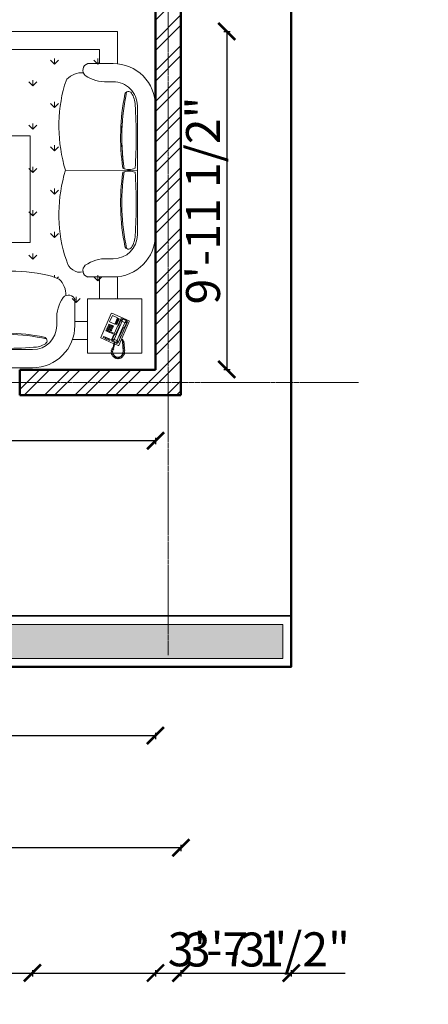
# Model space of a CAD drawing. Units: inches. Extents: x 261 to 2725, y 291 to 1454.
# Tile 11 of 35: x 898 to 1043, y 293 to 641. Entities that reach past the tile are written whole.
import ezdxf

# ---------------------------------------------------------------- set-up
doc = ezdxf.new("R2010")
doc.units = ezdxf.units.IN
doc.linetypes.add('CENTER', pattern=[2, 1.25, -0.25, 0.25, -0.25])
for name, color, linetype, lineweight in [('A-ANNO-DIMS', 136, 'Continuous', 18), ('A-FURN', 30, 'Continuous', 18), ('A-GRID', 251, 'CENTER', 13), ('A-PLNT', 3, 'Continuous', 18), ('A-PLNT-PATT', 3, 'Continuous', 13), ('A-WALL', 222, 'Continuous', 50), ('A-WALL-PATT', 243, 'Continuous', 13), ('C-PROP', 7, 'Continuous', 35)]:
    doc.layers.add(name, color=color, linetype=linetype, lineweight=lineweight)
doc.styles.get("Standard").update_dxf_attribs({"font": 'arial.ttf'})
doc.dimstyles.new('ISO-25', dxfattribs={"dimtxt": 12, "dimasz": 6, "dimexe": 1.25, "dimexo": 0.625, "dimtad": 1, "dimdec": 0, "dimlunit": 3, "dimtxsty": 'Standard', "dimblk": 'ARCHTICK', "dimcen": 2.5, "dimadec": 0, "dimazin": 0, "dimtfac": 1, "dimtdec": 0, "dimtmove": 0, "dimatfit": 3, "dimfxl": 1, "dimfxlon": 1, "dimarcsym": 0})

# ---------------------------------------------------------------- blocks, each defined once
blk = doc.blocks.new('A$C29956593')
for p, q in [((1017.8, 2786), (2742.6, 2786)), ((278.2, 2702.6), (273.3, 2697.8)), ((273.3, 2697.8), (276.9, 2686.9)), ((285.5, 2696.3), (278.2, 2702.6)), ((283.9, 2691.1), (302.3, 2697.9)), ((290.3, 2707.8), (284.9, 2706)), ((284.9, 2706), (285.5, 2696.3)), ((296.9, 2700.7), (290.3, 2707.8)), ((303.3, 2712.1), (296.9, 2710.1)), ((296.9, 2710.1), (296.9, 2700.7)), ((302.3, 2697.9), (322.4, 2697.8)), ((306.1, 2701.8), (303.3, 2712.1)), ((309.1, 2711), (306.1, 2701.8)), ((314.8, 2711.2), (309.1, 2711)), ((318.9, 2702.4), (314.8, 2711.2)), ((322.6, 2710.2), (318.9, 2702.4)), ((322.4, 2697.8), (339.2, 2688.6)), ((328.8, 2709.2), (322.6, 2710.2)), ((327.9, 2698.5), (328.8, 2709.2)), ((333.7, 2706), (327.9, 2698.5)), ((338.4, 2703.2), (333.7, 2706)), ((338.4, 2693.8), (338.4, 2703.2)), ((345.6, 2700), (338.4, 2693.8)), ((351, 2695.6), (345.6, 2700)), ((345.9, 2686.3), (351, 2695.6)), ((869.5, 2753), (870.7, 2751.8)), ((113, 2666.3), (113, 2216.3)), ((563, 2666.3), (113, 2666.3)), ((255.7, 2654.1), (254.5, 2644.2)), ((254.5, 2644.2), (263.6, 2641.2)), ((263.6, 2641.2), (254.7, 2635.1)), ((254.7, 2635.1), (255.8, 2629)), ((265.6, 2653.6), (255.7, 2654.1)), ((255.8, 2629), (265, 2627.7)), ((257.1, 2665), (256.2, 2657.4)), ((256.2, 2657.4), (265.6, 2653.6)), ((265.8, 2668.1), (257.1, 2665)), ((265, 2627.7), (257.1, 2621.8)), ((257.1, 2621.8), (257.6, 2614.3)), ((257.6, 2614.3), (266.7, 2613.4)), ((259.7, 2679.5), (257.9, 2671.6)), ((257.9, 2671.6), (265.8, 2668.1)), ((266.7, 2613.4), (258.5, 2609)), ((269.9, 2678.1), (259.7, 2679.5)), ((268, 2691.2), (264.2, 2685.9)), ((264.2, 2685.9), (269.9, 2678.1)), ((267.7, 2639.4), (270.2, 2671)), ((269.6, 2618.4), (267.7, 2639.4)), ((267.7, 2616.4), (269.6, 2618.4)), ((269.4, 2615), (267.7, 2616.4)), ((276.9, 2686.9), (268, 2691.2)), ((270.3, 2600.3), (269.4, 2615)), ((270.2, 2671), (283.9, 2691.1)), ((339.2, 2688.6), (351, 2673.6)), ((345.1, 2616), (342.8, 2608.6)), ((349.3, 2635.7), (345.1, 2629.6)), ((345.1, 2629.6), (348.7, 2623.5)), ((348.7, 2623.5), (345.1, 2616)), ((355.4, 2689.1), (345.9, 2686.3)), ((346.5, 2598), (349, 2613.2)), ((349, 2613.2), (352.7, 2620.7)), ((355.9, 2654.7), (349.3, 2635.7)), ((351, 2673.6), (355.9, 2654.7)), ((352.6, 2622.8), (357.2, 2624.6)), ((352.7, 2620.7), (352.6, 2622.8)), ((353.1, 2636.5), (363.4, 2637.8)), ((360.9, 2631.3), (353.1, 2636.5)), ((354.8, 2675.8), (359.4, 2683.1)), ((363.7, 2677.8), (354.8, 2675.8)), ((359.4, 2683.1), (355.4, 2689.1)), ((357.2, 2624.6), (360.9, 2631.3)), ((357.4, 2651), (368.4, 2653.8)), ((366.3, 2646), (357.4, 2651)), ((358, 2664.3), (365.7, 2670.6)), ((367.5, 2662.1), (358, 2664.3)), ((363.4, 2637.8), (366.3, 2646)), ((365.7, 2670.6), (363.7, 2677.8)), ((368.4, 2653.8), (367.5, 2662.1)), ((563, 2216.3), (563, 2666.3)), ((2910.7, 2636), (1017.8, 2636)), ((216.6, 2403), (304.3, 2601.6)), ((231.9, 2406.6), (308.2, 2579.2)), ((258.5, 2609), (258.5, 2601.3)), ((258.5, 2601.3), (267.9, 2601.3)), ((267.9, 2601.3), (258.9, 2597.3)), ((258.9, 2597.3), (259.1, 2591.7)), ((259.1, 2591.7), (268.7, 2590.5)), ((268.7, 2590.5), (260.3, 2584.2)), ((260.3, 2584.2), (260.7, 2578.8)), ((260.7, 2578.8), (269.3, 2577.7)), ((261.3, 2572.2), (261.1, 2568.5)), ((261.1, 2568.5), (263.9, 2566.2)), ((269.3, 2577.7), (261.3, 2572.2)), ((263.9, 2566.2), (269, 2563.6)), ((269, 2563.6), (270.6, 2556.3)), ((269.2, 2568), (274, 2569.4)), ((272.1, 2566.8), (269.2, 2568)), ((272.6, 2580.5), (270.3, 2600.3)), ((270.6, 2556.3), (273.2, 2552.7)), ((273.1, 2564.2), (272.1, 2566.8)), ((274, 2569.4), (272.6, 2580.5)), ((275.7, 2559.9), (273.1, 2564.2)), ((273.2, 2552.7), (280.8, 2548.3)), ((277.9, 2556.2), (275.7, 2559.9)), ((282.7, 2552.6), (277.9, 2556.2)), ((283.4, 2480.1), (317.7, 2557.8)), ((365, 2555.9), (288, 2381.8)), ((293.3, 2537.7), (293, 2529.2)), ((310.5, 2576.5), (293.3, 2537.7)), ((304.3, 2601.6), (308.5, 2603.2)), ((306.4, 2470), (340.7, 2547.7)), ((308.2, 2579.2), (319.2, 2584.7)), ((308.5, 2603.2), (339.5, 2589.5)), ((314.4, 2581.6), (310.5, 2576.5)), ((310.5, 2576.5), (317.7, 2557.8)), ((321.5, 2581.9), (314.4, 2581.6)), ((317.7, 2557.8), (320.4, 2560.1)), ((319.2, 2584.7), (336.1, 2577.2)), ((320.4, 2560.1), (321.5, 2581.9)), ((320.4, 2560.1), (340.5, 2551.2)), ((335.5, 2575.7), (321.5, 2581.9)), ((338.2, 2583.2), (333.9, 2571.3)), ((333.9, 2571.3), (338.3, 2569.4)), ((340.3, 2593.4), (338.2, 2583.2)), ((338.3, 2569.4), (343.5, 2581.9)), ((356, 2566.7), (340.1, 2573.7)), ((342.8, 2608.6), (340.3, 2593.4)), ((340.5, 2551.2), (356, 2566.7)), ((340.7, 2547.7), (340.5, 2551.2)), ((340.7, 2575.2), (360.9, 2566.2)), ((359.4, 2554.9), (340.7, 2547.7)), ((359.4, 2554.9), (342.2, 2516)), ((343.5, 2581.9), (346.5, 2598)), ((344.5, 2587.2), (452.3, 2539.6)), ((356, 2566.7), (360.5, 2561.3)), ((360.5, 2561.3), (359.4, 2554.9)), ((360.9, 2566.2), (365, 2555.9)), ((453.9, 2535.4), (366.2, 2336.9)), ((378.8, 2560), (375, 2551.4)), ((375, 2551.4), (389.4, 2545)), ((393.2, 2553.7), (378.8, 2560)), ((389.4, 2545), (393.2, 2553.7)), ((399, 2551.1), (395.2, 2542.5)), ((395.2, 2542.5), (409.6, 2536.1)), ((413.4, 2544.8), (399, 2551.1)), ((409.6, 2536.1), (413.4, 2544.8)), ((419.1, 2542.2), (415.3, 2533.6)), ((415.3, 2533.6), (429.7, 2527.2)), ((433.5, 2535.9), (419.1, 2542.2)), ((429.7, 2527.2), (433.5, 2535.9)), ((452.3, 2539.6), (453.9, 2535.4)), ((688, 2553), (563, 2553)), ((253.3, 2447), (259.3, 2452.9)), ((283.4, 2480.1), (254.8, 2415.4)), ((259.3, 2452.9), (266.8, 2458.2)), ((266.8, 2458.2), (272.7, 2467.7)), ((272.7, 2467.7), (279, 2482.1)), ((306.4, 2470), (277.8, 2405.2)), ((291.1, 2509.4), (279, 2482.1)), ((294.1, 2520.1), (291.1, 2509.4)), ((293, 2529.2), (294.1, 2520.1)), ((301.3, 2443), (304.3, 2453.7)), ((304.3, 2453.7), (310.7, 2468.1)), ((322.8, 2495.4), (310.7, 2468.1)), ((328.7, 2504.8), (322.8, 2495.4)), ((336.2, 2510.1), (328.7, 2504.8)), ((342.2, 2516), (336.2, 2510.1)), ((348.6, 2441), (352.4, 2449.6)), ((349.4, 2497.4), (353.2, 2506)), ((360.9, 2492.3), (349.4, 2497.4)), ((352.4, 2449.6), (361, 2445.8)), ((353.2, 2506), (364.8, 2500.9)), ((355.6, 2456.8), (359.4, 2465.5)), ((364.2, 2453), (355.6, 2456.8)), ((359.4, 2465.5), (368, 2461.6)), ((364.8, 2500.9), (360.9, 2492.3)), ((362.6, 2472.7), (366.4, 2481.3)), ((371.2, 2468.8), (362.6, 2472.7)), ((368, 2461.6), (364.2, 2453)), ((366.4, 2481.3), (375, 2477.5)), ((369.6, 2488.5), (373.4, 2497.1)), ((378.2, 2484.7), (369.6, 2488.5)), ((370, 2450.5), (373.8, 2459.1)), ((378.6, 2446.7), (370, 2450.5)), ((375, 2477.5), (371.2, 2468.8)), ((373.4, 2497.1), (382, 2493.3)), ((373.8, 2459.1), (382.4, 2455.3)), ((377, 2466.3), (380.8, 2474.9)), ((385.6, 2462.5), (377, 2466.3)), ((382, 2493.3), (378.2, 2484.7)), ((382.4, 2455.3), (378.6, 2446.7)), ((380.8, 2474.9), (389.4, 2471.1)), ((384, 2482.1), (387.8, 2490.7)), ((392.6, 2478.3), (384, 2482.1)), ((384.4, 2444.1), (388.2, 2452.7)), ((389.4, 2471.1), (385.6, 2462.5)), ((387.8, 2490.7), (396.4, 2486.9)), ((388.2, 2452.7), (396.8, 2448.9)), ((391.4, 2459.9), (395.2, 2468.6)), ((400, 2456.1), (391.4, 2459.9)), ((396.4, 2486.9), (392.6, 2478.3)), ((396.8, 2448.9), (393, 2440.3)), ((395.2, 2468.6), (403.8, 2464.8)), ((398.3, 2475.8), (402.2, 2484.4)), ((407, 2471.9), (398.3, 2475.8)), ((403.8, 2464.8), (400, 2456.1)), ((402.2, 2484.4), (410.8, 2480.6)), ((410.8, 2480.6), (407, 2471.9)), ((218.2, 2398.9), (216.6, 2403)), ((362.1, 2335.3), (218.2, 2398.9)), ((236, 2396.2), (231.9, 2406.6)), ((235, 2401.8), (236.1, 2408.2)), ((239.5, 2396.4), (235, 2401.8)), ((279.1, 2377.1), (236, 2396.2)), ((236.1, 2408.2), (253.3, 2447)), ((236.1, 2408.2), (254.8, 2415.4)), ((254.9, 2411.9), (239.5, 2396.4)), ((274, 2381.1), (239.5, 2396.4)), ((254.8, 2415.4), (254.9, 2411.9)), ((254.9, 2411.9), (275.1, 2403)), ((275.1, 2403), (274, 2381.1)), ((274, 2381.1), (281, 2381.5)), ((277.8, 2405.2), (275.1, 2403)), ((285, 2386.6), (277.8, 2405.2)), ((288, 2381.8), (279.1, 2377.1)), ((281, 2381.5), (285, 2386.6)), ((285, 2386.6), (302.2, 2425.4)), ((301.9, 2386), (300, 2381.7)), ((300, 2381.7), (311.5, 2376.6)), ((302.5, 2433.9), (301.3, 2443)), ((313.4, 2380.9), (301.9, 2386)), ((302.2, 2425.4), (302.5, 2433.9)), ((305.7, 2394.6), (303.8, 2390.3)), ((303.8, 2390.3), (315.3, 2385.2)), ((317.3, 2389.5), (305.7, 2394.6)), ((309.6, 2403.2), (307.6, 2398.9)), ((307.6, 2398.9), (319.2, 2393.8)), ((321.1, 2398.1), (309.6, 2403.2)), ((313.4, 2411.9), (311.5, 2407.5)), ((311.5, 2407.5), (323, 2402.5)), ((311.5, 2376.6), (313.4, 2380.9)), ((324.9, 2406.8), (313.4, 2411.9)), ((314.6, 2371.8), (338.1, 2425)), ((356.3, 2353.3), (314.6, 2371.8)), ((317.2, 2420.5), (315.3, 2416.2)), ((315.3, 2416.2), (326.8, 2411.1)), ((315.3, 2385.2), (317.3, 2389.5)), ((328.7, 2415.4), (317.2, 2420.5)), ((321, 2429.1), (319.1, 2424.8)), ((319.1, 2424.8), (330.6, 2419.7)), ((319.2, 2393.8), (321.1, 2398.1)), ((332.5, 2424), (321, 2429.1)), ((323, 2402.5), (324.9, 2406.8)), ((326.8, 2411.1), (328.7, 2415.4)), ((330.6, 2419.7), (332.5, 2424)), ((338.1, 2425), (379.8, 2406.6)), ((357.2, 2437.2), (348.6, 2441)), ((379.8, 2406.6), (356.3, 2353.3)), ((361, 2445.8), (357.2, 2437.2)), ((363, 2434.6), (366.8, 2443.3)), ((371.6, 2430.8), (363, 2434.6)), ((366.8, 2443.3), (375.4, 2439.5)), ((375.4, 2439.5), (371.6, 2430.8)), ((377.4, 2428.3), (381.2, 2436.9)), ((386, 2424.5), (377.4, 2428.3)), ((381.2, 2436.9), (389.8, 2433.1)), ((393, 2440.3), (384.4, 2444.1)), ((389.8, 2433.1), (386, 2424.5)), ((667.8, 2403), (563, 2403)), ((667.8, 2436), (667.8, 2224.3)), ((817.8, 2436), (817.8, 2388.1)), ((366.2, 2336.9), (362.1, 2335.3)), ((113, 2216.3), (563, 2216.3)), ((314.4, 2216.3), (314.4, 2031.9)), ((328.6, 2216.3), (331.9, 2213)), ((464.4, 2216.3), (464.4, 2033.7)), ((657.5, 2246.7), (623.8, 2213)), ((657.5, 2246.7), (691.1, 2213)), ((657.5, 2246.7), (657.5, 2199.1)), ((477.8, 2067.1), (444.2, 2033.4)), ((477.8, 2067.1), (511.5, 2033.4)), ((477.9, 2067.1), (477.9, 2019.5)), ((798.2, 2052), (847, 2032.1)), ((815.1, 2045.1), (803.4, 2033.4)), ((350, 2033.7), (561.7, 2033.7)), ((837.1, 2036.1), (837.1, 2019.5)), ((350, 1883.7), (397.8, 1883.7)), ((755.2, 1851.4), (733.9, 1903.4)), ((1016.7, 1887.5), (983, 1853.8)), ((1016.7, 1887.5), (1016.7, 1839.9)), ((1016.7, 1887.5), (1050.3, 1853.8)), ((1039.5, 1747.2), (2898.7, 1747.2)), ((1039.5, 864.7), (1039.5, 1747.2)), ((0, 1683.7), (0, 783.9)), ((150, 615.8), (150, 1683.7)), ((837.1, 1707.9), (803.4, 1674.2)), ((837.1, 1707.9), (870.7, 1674.2)), ((837.1, 1707.9), (837.1, 1660.3)), ((1016.7, 1528.3), (983, 1494.6)), ((1016.7, 1528.3), (1050.3, 1494.6)), ((1016.7, 1528.3), (1016.7, 1480.6)), ((837.1, 1348.7), (803.4, 1315)), ((837.1, 1348.7), (870.7, 1315)), ((837.1, 1348.7), (837.1, 1301)), ((745.9, 1150.3), (150, 1150.5)), ((1016.7, 1169), (983, 1135.4)), ((1016.7, 1169.1), (1016.7, 1121.4)), ((1016.7, 1169), (1050.3, 1135.4)), ((837.1, 989.4), (803.4, 955.8)), ((837.1, 989.5), (837.1, 941.8)), ((837.1, 989.4), (870.7, 955.8)), ((2898.7, 864.7), (1039.5, 864.7)), ((0, 783.9), (0, 615.8)), ((1016.7, 809.8), (983, 776.2)), ((1016.7, 809.9), (1016.7, 762.2)), ((1016.7, 809.8), (1050.3, 776.2)), ((837.1, 630.2), (803.4, 596.6)), ((837.1, 630.2), (837.1, 582.6)), ((837.1, 630.2), (870.7, 596.6)), ((397.8, 415.8), (350, 415.8)), ((733.9, 396.1), (753.9, 445)), ((1016.7, 450.6), (983, 417)), ((1016.7, 450.6), (1016.7, 403)), ((1016.7, 450.6), (1050.3, 417)), ((314.4, 267.6), (314.4, 0)), ((350, 265.8), (561.7, 265.8)), ((464.4, 265.8), (464.4, 150)), ((472.6, 265.8), (464.4, 257.6)), ((477.8, 271), (472.6, 265.8)), ((477.8, 271), (483.1, 265.8)), ((477.9, 271), (477.9, 265.8)), ((477.9, 265.8), (477.9, 223.4)), ((483.1, 265.8), (511.5, 237.3)), ((837.1, 271), (803.4, 237.3)), ((837.1, 271), (870.7, 237.3)), ((837.1, 271), (837.1, 223.4)), ((464.4, 150), (3537.6, 150)), ((314.4, 0), (3687.6, 0))]:
    blk.add_line(p, q)
for centre, radius, start, end in [((1017.8, 2436), 350, 89.99998, 179.99998), ((1017.8, 2436), 200, 89.99998, 179.99998), ((1011.2, 2436.9), 180, 89.99998, 123.49883), ((1272.9, -801.2), 3428.1, 85.62178, 94.37818), ((928.5, 2562), 30, 123.49883, 258.53473), ((1278, 4285.1), 1778.2, 257.81016, 278.43024), ((1278, 4285.1), 1788.2, 258.53473, 278.25333), ((534.8, 2371.7), 283.5, 323.90077, 3.32258), ((720.5, 2241.4), 56.8, 197.47273, 319.7773), ((918.2, 2179.8), 175.3, 177.10657, 226.78661), ((1184.5, 3255.7), 1269.7, 254.72966, 286.78715), ((350, 1683.7), 350, 90.00002, 180.00002), ((544.6, 1981), 56.8, 310.2227, 72.52727), ((624.3, 1883.4), 111.5, 10.33151, 102.42525), ((350, 1683.7), 200, 90.00002, 180.00002), ((414.3, 2166.7), 283.5, 266.67742, 306.09923), ((224, 1773), 30, 11.46527, 146.50117), ((-1499.2, 1423.6), 1778.2, 351.56976, 12.18984), ((-469.7, 1517), 1269.7, 343.21285, 15.27034), ((349.1, 1690.3), 180, 146.50117, 180.00002), ((-1499.2, 1423.6), 1788.2, 351.74667, 11.46527), ((3587.2, 1428.6), 3428.1, 175.62182, 184.37822), ((219.8, 1286.3), 129.8, 246.98328, 293.01676), ((219.8, 1013.2), 129.8, 66.98324, 113.01672), ((-468.2, 783.8), 1268.2, 344.4627, 16.79693), ((3587.2, 870.9), 3428.1, 175.62178, 184.37818), ((-1499.2, 875.9), 1778.2, 347.81016, 8.43024), ((-1499.2, 875.9), 1788.2, 348.53473, 8.25333), ((-2891.8, 790.6), 3171.8, 359.87755, 6.30976), ((350, 615.8), 350, 179.99998, 269.99998), ((350, 615.8), 200, 179.99998, 269.99998), ((349.1, 609.2), 180, 179.99998, 213.49883), ((224, 526.4), 30, 213.49883, 348.53473), ((419.8, 145.5), 271.2, 53.45039, 94.64105), ((544.6, 320), 56.8, 287.47277, 49.77733), ((606.2, 516.1), 175.3, 267.10659, 316.78663)]:
    blk.add_arc(centre, radius, start, end)
blk = doc.blocks.new('_ArchTick')
at = {"color": 0, "linetype": 'ByBlock', "const_width": 0.15}
blk.add_lwpolyline([(-0.5, -0.5), (0.5, 0.5)], dxfattribs=at)
blk = doc.blocks.new('*D28')
at = {"layer": 'A-ANNO-DIMS', "color": 0, "lineweight": -2, "transparency": 16777216}
for p, q in [((469.45, 349.55), (469.45, 347.3)), ((469.45, 348.55), (955.45, 348.55)), ((955.45, 349.55), (955.45, 347.3))]:
    blk.add_line(p, q, dxfattribs=at)
at = {"layer": 'Defpoints', "color": 0, "transparency": 16777216}
for p in [(469.45, 508.47), (955.45, 508.47), (955.45, 348.55)]:
    blk.add_point(p, dxfattribs=at)
at = {"layer": 'A-ANNO-DIMS', "color": 0, "lineweight": -2, "transparency": 16777216, "xscale": 6, "yscale": 6, "zscale": 6, "rotation": 180}
blk.add_blockref('_ArchTick', (469.45, 348.55), dxfattribs=at)
at = {"layer": 'A-ANNO-DIMS', "color": 0, "lineweight": -2, "transparency": 16777216, "xscale": 6, "yscale": 6, "zscale": 6}
blk.add_blockref('_ArchTick', (955.45, 348.55), dxfattribs=at)
at = {"layer": 'A-ANNO-DIMS', "color": 0, "transparency": 16777216, "insert": (712.45, 355.3), "char_height": 12, "attachment_point": 5}
blk.add_mtext('40\'-6"', dxfattribs=at)
blk = doc.blocks.new('*D31')
at = {"layer": 'A-ANNO-DIMS', "color": 0, "lineweight": -2, "transparency": 16777216}
for p, q in [((478.45, 389.14), (478.45, 386.89)), ((478.45, 388.14), (946.45, 388.14)), ((946.45, 389.14), (946.45, 386.89))]:
    blk.add_line(p, q, dxfattribs=at)
at = {"layer": 'Defpoints', "color": 0, "transparency": 16777216}
for p in [(478.45, 517.47), (946.45, 517.47), (946.45, 388.14)]:
    blk.add_point(p, dxfattribs=at)
at = {"layer": 'A-ANNO-DIMS', "color": 0, "lineweight": -2, "transparency": 16777216, "xscale": 6, "yscale": 6, "zscale": 6, "rotation": 180}
blk.add_blockref('_ArchTick', (478.45, 388.14), dxfattribs=at)
at = {"layer": 'A-ANNO-DIMS', "color": 0, "lineweight": -2, "transparency": 16777216, "xscale": 6, "yscale": 6, "zscale": 6}
blk.add_blockref('_ArchTick', (946.45, 388.14), dxfattribs=at)
at = {"layer": 'A-ANNO-DIMS', "color": 0, "transparency": 16777216, "insert": (712.45, 394.89), "char_height": 12, "attachment_point": 5}
blk.add_mtext("39'", dxfattribs=at)
blk = doc.blocks.new('*D67')
at = {"layer": 'A-ANNO-DIMS', "color": 0, "lineweight": -2, "ltscale": 0.07, "transparency": 16777216}
for p, q in [((778.45, 492.4), (526.52, 492.4)), ((778.45, 493.4), (778.45, 491.15)), ((946.45, 492.4), (778.45, 492.4)), ((946.45, 493.4), (946.45, 491.15))]:
    blk.add_line(p, q, dxfattribs=at)
at = {"layer": 'Defpoints', "color": 0, "ltscale": 0.07, "transparency": 16777216}
for p in [(778.45, 517.6), (946.45, 517.6), (778.45, 492.4)]:
    blk.add_point(p, dxfattribs=at)
at = {"layer": 'A-ANNO-DIMS', "color": 0, "lineweight": -2, "ltscale": 0.07, "transparency": 16777216, "xscale": 6, "yscale": 6, "zscale": 6, "rotation": 180}
blk.add_blockref('_ArchTick', (778.45, 492.4), dxfattribs=at)
at = {"layer": 'A-ANNO-DIMS', "color": 0, "lineweight": -2, "ltscale": 0.07, "transparency": 16777216, "xscale": 6, "yscale": 6, "zscale": 6}
blk.add_blockref('_ArchTick', (946.45, 492.4), dxfattribs=at)
at = {"layer": 'A-ANNO-DIMS', "color": 0, "ltscale": 0.07, "transparency": 16777216, "insert": (649.49, 499.24), "char_height": 12, "attachment_point": 5}
blk.add_mtext('LIVING ROOM SOFA SET 14\'-0"', dxfattribs=at)
blk = doc.blocks.new('*D68')
at = {"layer": 'A-ANNO-DIMS', "color": 0, "lineweight": -2, "ltscale": 0.07, "transparency": 16777216}
for p, q in [((970.65, 637.08), (972.9, 637.08)), ((971.65, 637.08), (971.65, 517.6)), ((970.65, 517.6), (972.9, 517.6))]:
    blk.add_line(p, q, dxfattribs=at)
at = {"layer": 'Defpoints', "color": 0, "ltscale": 0.07, "transparency": 16777216}
for p in [(946.45, 637.08), (946.45, 517.6), (971.65, 517.6)]:
    blk.add_point(p, dxfattribs=at)
at = {"layer": 'A-ANNO-DIMS', "color": 0, "lineweight": -2, "ltscale": 0.07, "transparency": 16777216, "xscale": 6, "yscale": 6, "zscale": 6}
for p, rotation in [((971.65, 637.08), 90), ((971.65, 517.6), 270)]:
    blk.add_blockref('_ArchTick', p, dxfattribs=dict(at, rotation=rotation))
at = {"layer": 'A-ANNO-DIMS', "color": 0, "ltscale": 0.07, "transparency": 16777216, "insert": (964.82, 577.34), "char_height": 12, "attachment_point": 5, "rotation": 90}
blk.add_mtext('9\'-11 1/2"', dxfattribs=at)
blk = doc.blocks.new('*D82')
at = {"layer": 'A-ANNO-DIMS', "color": 0, "lineweight": -2, "ltscale": 0.07, "transparency": 16777216}
for p, q in [((2600.96, 679.47), (2603.21, 679.47)), ((2601.96, 517.47), (2601.96, 679.47)), ((2600.96, 517.47), (2603.21, 517.47))]:
    blk.add_line(p, q, dxfattribs=at)
at = {"layer": 'Defpoints', "color": 0, "ltscale": 0.07, "transparency": 16777216}
for p in [(946.45, 679.47), (2601.96, 679.47), (946.45, 517.47)]:
    blk.add_point(p, dxfattribs=at)
at = {"layer": 'A-ANNO-DIMS', "color": 0, "lineweight": -2, "ltscale": 0.07, "transparency": 16777216, "xscale": 6, "yscale": 6, "zscale": 6}
for p, rotation in [((2601.96, 679.47), 90), ((2601.96, 517.47), 270)]:
    blk.add_blockref('_ArchTick', p, dxfattribs=dict(at, rotation=rotation))
at = {"layer": 'A-ANNO-DIMS', "color": 0, "ltscale": 0.07, "transparency": 16777216, "insert": (2595.2, 598.47), "char_height": 12, "attachment_point": 5, "rotation": 90}
blk.add_mtext('13\'-6"', dxfattribs=at)
blk = doc.blocks.new('*D88')
at = {"layer": 'A-ANNO-DIMS', "color": 0, "lineweight": -2, "ltscale": 0.07, "transparency": 16777216}
for p, q in [((430.45, 305.22), (430.45, 302.97)), ((430.45, 304.22), (994.45, 304.22)), ((994.45, 305.22), (994.45, 302.97))]:
    blk.add_line(p, q, dxfattribs=at)
at = {"layer": 'Defpoints', "color": 0, "ltscale": 0.07, "transparency": 16777216}
for p in [(430.45, 412.47), (994.45, 412.47), (994.45, 304.22)]:
    blk.add_point(p, dxfattribs=at)
at = {"layer": 'A-ANNO-DIMS', "color": 0, "lineweight": -2, "ltscale": 0.07, "transparency": 16777216, "xscale": 6, "yscale": 6, "zscale": 6, "rotation": 180}
blk.add_blockref('_ArchTick', (430.45, 304.22), dxfattribs=at)
at = {"layer": 'A-ANNO-DIMS', "color": 0, "lineweight": -2, "ltscale": 0.07, "transparency": 16777216, "xscale": 6, "yscale": 6, "zscale": 6}
blk.add_blockref('_ArchTick', (994.45, 304.22), dxfattribs=at)
at = {"layer": 'A-ANNO-DIMS', "color": 0, "ltscale": 0.07, "transparency": 16777216, "insert": (712.45, 310.97), "char_height": 12, "attachment_point": 5}
blk.add_mtext('47\'-0"', dxfattribs=at)
blk = doc.blocks.new('*D89')
at = {"layer": 'A-ANNO-DIMS', "color": 0, "lineweight": -2, "ltscale": 0.07, "transparency": 16777216}
for p, q in [((2600.96, 508.47), (2603.21, 508.47)), ((2601.96, 412.47), (2601.96, 508.47)), ((2600.96, 412.47), (2603.21, 412.47))]:
    blk.add_line(p, q, dxfattribs=at)
at = {"layer": 'Defpoints', "color": 0, "ltscale": 0.07, "transparency": 16777216}
for p in [(955.45, 508.47), (2601.96, 508.47), (994.45, 412.47)]:
    blk.add_point(p, dxfattribs=at)
at = {"layer": 'A-ANNO-DIMS', "color": 0, "lineweight": -2, "ltscale": 0.07, "transparency": 16777216, "xscale": 6, "yscale": 6, "zscale": 6}
for p, rotation in [((2601.96, 508.47), 90), ((2601.96, 412.47), 270)]:
    blk.add_blockref('_ArchTick', p, dxfattribs=dict(at, rotation=rotation))
at = {"layer": 'A-ANNO-DIMS', "color": 0, "ltscale": 0.07, "transparency": 16777216, "insert": (2595.21, 460.47), "char_height": 12, "attachment_point": 5, "rotation": 90}
blk.add_mtext('8\'-0"', dxfattribs=at)
blk = doc.blocks.new('*D92')
at = {"layer": 'A-ANNO-DIMS', "color": 0, "lineweight": -2, "ltscale": 0.07, "transparency": 16777216}
for p, q in [((955.45, 305.22), (955.45, 302.97)), ((955.45, 304.22), (994.45, 304.22)), ((994.45, 305.22), (994.45, 302.97))]:
    blk.add_line(p, q, dxfattribs=at)
at = {"layer": 'Defpoints', "color": 0, "ltscale": 0.07, "transparency": 16777216}
for p in [(955.45, 508.47), (994.45, 430.47), (994.45, 304.22)]:
    blk.add_point(p, dxfattribs=at)
at = {"layer": 'A-ANNO-DIMS', "color": 0, "lineweight": -2, "ltscale": 0.07, "transparency": 16777216, "xscale": 6, "yscale": 6, "zscale": 6, "rotation": 180}
blk.add_blockref('_ArchTick', (955.45, 304.22), dxfattribs=at)
at = {"layer": 'A-ANNO-DIMS', "color": 0, "lineweight": -2, "ltscale": 0.07, "transparency": 16777216, "xscale": 6, "yscale": 6, "zscale": 6}
blk.add_blockref('_ArchTick', (994.45, 304.22), dxfattribs=at)
at = {"layer": 'A-ANNO-DIMS', "color": 0, "ltscale": 0.07, "transparency": 16777216, "insert": (974.95, 310.97), "char_height": 12, "attachment_point": 5}
blk.add_mtext('3\'-3"', dxfattribs=at)
blk = doc.blocks.new('*D101')
at = {"layer": 'A-ANNO-DIMS', "color": 0, "lineweight": -2, "ltscale": 0.07, "transparency": 16777216}
for p, q in [((902.95, 305.22), (902.95, 302.97)), ((902.95, 304.22), (946.45, 304.22)), ((946.45, 305.22), (946.45, 302.97)), ((946.45, 304.22), (1013.55, 304.22))]:
    blk.add_line(p, q, dxfattribs=at)
at = {"layer": 'Defpoints', "color": 0, "ltscale": 0.07, "transparency": 16777216}
for p in [(902.95, 679.47), (946.45, 679.47), (946.45, 304.22)]:
    blk.add_point(p, dxfattribs=at)
at = {"layer": 'A-ANNO-DIMS', "color": 0, "lineweight": -2, "ltscale": 0.07, "transparency": 16777216, "xscale": 6, "yscale": 6, "zscale": 6, "rotation": 180}
blk.add_blockref('_ArchTick', (902.95, 304.22), dxfattribs=at)
at = {"layer": 'A-ANNO-DIMS', "color": 0, "lineweight": -2, "ltscale": 0.07, "transparency": 16777216, "xscale": 6, "yscale": 6, "zscale": 6}
blk.add_blockref('_ArchTick', (946.45, 304.22), dxfattribs=at)
at = {"layer": 'A-ANNO-DIMS', "color": 0, "ltscale": 0.07, "transparency": 16777216, "insert": (983, 311.05), "char_height": 12, "attachment_point": 5}
blk.add_mtext('3\'-7 1/2"', dxfattribs=at)
blk = doc.blocks.new('*D103')
at = {"layer": 'A-ANNO-DIMS', "color": 0, "lineweight": -2, "ltscale": 0.07, "transparency": 16777216}
for p, q in [((287.06, 1231.47), (284.81, 1231.47)), ((286.06, 439.47), (286.06, 1231.47)), ((287.06, 439.47), (284.81, 439.47))]:
    blk.add_line(p, q, dxfattribs=at)
at = {"layer": 'Defpoints', "color": 0, "ltscale": 0.07, "transparency": 16777216}
for p in [(286.06, 1231.47), (1243.08, 1231.47), (1243.08, 439.47)]:
    blk.add_point(p, dxfattribs=at)
at = {"layer": 'A-ANNO-DIMS', "color": 0, "lineweight": -2, "ltscale": 0.07, "transparency": 16777216, "xscale": 6, "yscale": 6, "zscale": 6}
for p, rotation in [((286.06, 1231.47), 90), ((286.06, 439.47), 270)]:
    blk.add_blockref('_ArchTick', p, dxfattribs=dict(at, rotation=rotation))
at = {"layer": 'A-ANNO-DIMS', "color": 0, "ltscale": 0.07, "transparency": 16777216, "insert": (279.3, 835.47), "char_height": 12, "attachment_point": 5, "rotation": 90}
blk.add_mtext('66\'-0"', dxfattribs=at)
blk = doc.blocks.new('*D106')
at = {"layer": 'A-ANNO-DIMS', "color": 0, "lineweight": -2, "ltscale": 0.07, "transparency": 16777216}
for p, q in [((287.06, 496.47), (284.81, 496.47)), ((286.06, 448.47), (286.06, 496.47)), ((287.06, 448.47), (284.81, 448.47))]:
    blk.add_line(p, q, dxfattribs=at)
at = {"layer": 'Defpoints', "color": 0, "ltscale": 0.07, "transparency": 16777216}
for p in [(286.06, 496.47), (1252.08, 496.47), (1252.08, 448.47)]:
    blk.add_point(p, dxfattribs=at)
at = {"layer": 'A-ANNO-DIMS', "color": 0, "lineweight": -2, "ltscale": 0.07, "transparency": 16777216, "xscale": 6, "yscale": 6, "zscale": 6}
for p, rotation in [((286.06, 496.47), 90), ((286.06, 448.47), 270)]:
    blk.add_blockref('_ArchTick', p, dxfattribs=dict(at, rotation=rotation))
at = {"layer": 'A-ANNO-DIMS', "color": 0, "ltscale": 0.07, "transparency": 16777216, "insert": (279.3, 472.47), "char_height": 12, "attachment_point": 5, "rotation": 90}
blk.add_mtext('4\'-0"', dxfattribs=at)
blk = doc.blocks.new('*D107')
at = {"layer": 'A-ANNO-DIMS', "color": 0, "lineweight": -2, "ltscale": 0.07, "transparency": 16777216}
for p, q in [((287.06, 673.47), (284.81, 673.47)), ((286.06, 496.47), (286.06, 673.47)), ((287.06, 496.47), (284.81, 496.47))]:
    blk.add_line(p, q, dxfattribs=at)
at = {"layer": 'Defpoints', "color": 0, "ltscale": 0.07, "transparency": 16777216}
for p in [(286.06, 673.47), (1252.08, 673.47), (1252.08, 496.47)]:
    blk.add_point(p, dxfattribs=at)
at = {"layer": 'A-ANNO-DIMS', "color": 0, "lineweight": -2, "ltscale": 0.07, "transparency": 16777216, "xscale": 6, "yscale": 6, "zscale": 6}
for p, rotation in [((286.06, 673.47), 90), ((286.06, 496.47), 270)]:
    blk.add_blockref('_ArchTick', p, dxfattribs=dict(at, rotation=rotation))
at = {"layer": 'A-ANNO-DIMS', "color": 0, "ltscale": 0.07, "transparency": 16777216, "insert": (279.3, 584.97), "char_height": 12, "attachment_point": 5, "rotation": 90}
blk.add_mtext('14\'-9"', dxfattribs=at)
blk = doc.blocks.new('*D123')
at = {"layer": 'A-ANNO-DIMS', "color": 0, "lineweight": -2, "ltscale": 0.07, "transparency": 16777216}
for p, q in [((287.06, 1054.85), (284.81, 1054.85)), ((286.06, 439.47), (286.06, 1054.85)), ((287.06, 439.47), (284.81, 439.47))]:
    blk.add_line(p, q, dxfattribs=at)
at = {"layer": 'Defpoints', "color": 0, "ltscale": 0.07, "transparency": 16777216}
for p in [(286.06, 1054.85), (2007.71, 1054.85), (2007.71, 439.47)]:
    blk.add_point(p, dxfattribs=at)
at = {"layer": 'A-ANNO-DIMS', "color": 0, "lineweight": -2, "ltscale": 0.07, "transparency": 16777216, "xscale": 6, "yscale": 6, "zscale": 6}
for p, rotation in [((286.06, 1054.85), 90), ((286.06, 439.47), 270)]:
    blk.add_blockref('_ArchTick', p, dxfattribs=dict(at, rotation=rotation))
at = {"layer": 'A-ANNO-DIMS', "color": 0, "ltscale": 0.07, "transparency": 16777216, "insert": (279.22, 747.16), "char_height": 12, "attachment_point": 5, "rotation": 90}
blk.add_mtext('51\'-3 1/2"', dxfattribs=at)

msp = doc.modelspace()

# ---------------------------------------------------------------- hatches: boundary and pattern name
at = {"layer": 'A-PLNT-PATT'}
h = msp.add_hatch(dxfattribs=at)
h.set_pattern_fill('GRASS', color=256, scale=0.7)
h.paths.add_polyline_path([(658.45, 427.47), (433.45, 427.47), (433.45, 415.47), (658.45, 415.47)])
h.paths.add_polyline_path([(670.45, 421.47), (664.45, 421.47), (664.45, 415.47), (670.45, 415.47)])
h.paths.add_polyline_path([(784.45, 421.47), (778.45, 421.47), (778.45, 415.47), (784.45, 415.47)])
h.paths.add_polyline_path([(991.45, 427.47), (790.45, 427.47), (790.45, 415.47), (991.45, 415.47)])
h.paths.add_polyline_path([(1439.08, 1220.47), (1252.08, 1220.47), (1252.08, 1198.47), (1417.08, 1198.47), (1417.08, 1117.47), (1439.08, 1117.47)])
h.paths.add_polyline_path([(2304.71, 1045.85), (2016.71, 1045.85), (2016.71, 805.87), (2304.71, 805.87)])
h.paths.add_polyline_path([(1267.21, 1201.68), (1431.59, 1201.68), (1431.59, 1218.76), (1267.21, 1218.76)], flags=24)
h.paths.add_polyline_path([(2089.2, 883.04), (2242.64, 883.04), (2242.64, 936.27), (2089.2, 936.27)], flags=24)
at = {"layer": 'A-WALL-PATT'}
h = msp.add_hatch(dxfattribs=at)
h.set_pattern_fill('ANSI32', color=256, scale=0.8)
h.paths.add_polyline_path([(478.45, 685.47), (580.45, 685.47), (580.45, 691.47), (577.45, 691.47), (577.45, 694.47), (571.45, 694.47), (571.45, 691.47), (478.45, 691.47), (478.45, 721.47), (469.45, 721.47), (469.45, 508.47), (538.45, 508.47), (538.45, 517.47), (478.45, 517.47)])
h.paths.add_polyline_path([(694.45, 517.47), (676.45, 517.47), (676.45, 646.47), (670.45, 646.47), (670.45, 517.47), (610.45, 517.47), (610.45, 508.47), (694.45, 508.47)])
h.paths.add_polyline_path([(676.45, 784.47), (478.45, 784.47), (478.45, 844.47), (469.45, 844.47), (469.45, 745.47), (478.45, 745.47), (478.45, 775.47), (571.45, 775.47), (571.45, 724.47), (577.45, 724.47), (577.45, 775.47), (670.45, 775.47), (670.45, 691.47), (610.45, 691.47), (610.45, 685.47), (670.45, 685.47), (670.45, 682.47), (676.45, 682.47)])
h.paths.add_polyline_path([(955.45, 880.47), (946.45, 880.47), (946.45, 808.47), (778.45, 808.47), (778.45, 799.47), (946.45, 799.47), (946.45, 517.47), (898.45, 517.47), (898.45, 508.47), (955.45, 508.47)])
h.paths.add_polyline_path([(778.45, 598.47), (772.45, 598.47), (772.45, 517.47), (754.45, 517.47), (754.45, 508.47), (826.45, 508.47), (826.45, 517.47), (778.45, 517.47)])
h.paths.add_polyline_path([(955.45, 1090.47), (946.45, 1090.47), (946.45, 1030.47), (817.45, 1030.47), (817.45, 1024.47), (946.45, 1024.47), (946.45, 952.47), (955.45, 952.47)])
h.paths.add_polyline_path([(955.45, 1231.47), (730.45, 1231.47), (730.45, 1222.47), (772.45, 1222.47), (772.45, 1096.47), (766.45, 1096.47), (766.45, 1090.47), (772.45, 1090.47), (772.45, 1006.47), (712.45, 1006.47), (712.45, 1000.47), (778.45, 1000.47), (778.45, 1024.47), (781.45, 1024.47), (781.45, 1030.47), (778.45, 1030.47), (778.45, 1222.47), (946.45, 1222.47), (946.45, 1162.47), (955.45, 1162.47)])
h.paths.add_polyline_path([(694.45, 1231.47), (619.45, 1231.47), (619.45, 1222.47), (646.45, 1222.47), (646.45, 1039.47), (652.45, 1039.47), (652.45, 1090.47), (736.45, 1090.47), (736.45, 1096.47), (652.45, 1096.47), (652.45, 1222.47), (694.45, 1222.47)])
h.paths.add_polyline_path([(571.45, 1231.47), (469.45, 1231.47), (469.45, 1099.47), (478.45, 1099.47), (478.45, 1144.47), (544.45, 1144.47), (544.45, 1153.47), (538.45, 1153.47), (538.45, 1150.47), (478.45, 1150.47), (478.45, 1222.47), (538.45, 1222.47), (538.45, 1183.47), (544.45, 1183.47), (544.45, 1222.47), (571.45, 1222.47)])
h.paths.add_polyline_path([(538.45, 1006.47), (478.45, 1006.47), (478.45, 1051.47), (469.45, 1051.47), (469.45, 940.47), (478.45, 940.47), (478.45, 1000.47), (538.45, 1000.47)])
h.paths.add_polyline_path([(652.45, 1006.47), (652.45, 1009.47), (646.45, 1009.47), (646.45, 1006.47), (586.45, 1006.47), (586.45, 1000.47), (652.45, 1000.47)])
h.paths.add_polyline_path([(1288.08, 973.47), (1243.08, 973.47), (1243.08, 920.97), (1252.08, 920.97), (1252.08, 964.47), (1288.08, 964.47)], flags=17)
h.paths.add_polyline_path([(1402.08, 805.47), (1252.08, 805.47), (1252.08, 848.97), (1243.08, 848.97), (1243.08, 757.47), (1252.08, 757.47), (1252.08, 799.47), (1294.08, 799.47), (1372.08, 799.47), (1372.08, 779.47), (1372.08, 715.47), (1378.08, 715.47), (1378.08, 799.47), (1402.08, 799.47)])
h.paths.add_polyline_path([(1252.08, 721.47), (1243.08, 721.47), (1243.08, 439.47), (1729.08, 439.47), (1729.08, 709.47), (1720.08, 709.47), (1720.08, 679.47), (1582.08, 679.47), (1582.08, 670.47), (1588.08, 670.47), (1588.08, 673.47), (1720.08, 673.47), (1720.08, 559.47), (1690.08, 559.47), (1690.08, 550.47), (1720.08, 550.47), (1720.08, 448.47), (1252.08, 448.47), (1252.08, 496.47), (1312.08, 496.47), (1312.08, 505.47), (1252.08, 505.47), (1252.08, 673.47), (1405.08, 673.47), (1405.08, 679.47), (1378.08, 679.47), (1378.08, 685.47), (1372.08, 685.47), (1372.08, 679.47), (1252.08, 679.47)])
h.paths.add_polyline_path([(1450.08, 550.47), (1480.08, 550.47), (1480.08, 559.47), (1450.08, 559.47), (1450.08, 679.47), (1441.08, 679.47), (1441.08, 673.47), (1444.08, 673.47), (1444.08, 505.47), (1384.08, 505.47), (1384.08, 496.47), (1450.08, 496.47)], flags=17)
h.paths.add_polyline_path([(1618.08, 559.47), (1588.08, 559.47), (1588.08, 634.47), (1582.08, 634.47), (1582.08, 559.47), (1552.08, 559.47), (1552.08, 550.47), (1618.08, 550.47)], flags=17)
h.paths.add_polyline_path([(1564.08, 964.47), (1630.08, 964.47), (1630.08, 973.47), (1477.08, 973.47), (1477.08, 964.47), (1558.08, 964.47), (1558.08, 926.22), (1558.08, 887.97), (1486.08, 887.97), (1486.08, 881.97), (1558.08, 881.97), (1558.08, 805.47), (1450.08, 805.47), (1450.08, 845.97), (1444.08, 845.97), (1444.08, 805.47), (1438.08, 805.47), (1438.08, 799.47), (1564.08, 799.47)], flags=17)
h.paths.add_polyline_path([(1453.08, 973.47), (1408.08, 973.47), (1408.08, 964.47), (1444.08, 964.47), (1444.08, 881.97), (1450.08, 881.97), (1456.08, 881.97), (1456.08, 887.97), (1450.08, 887.97), (1450.08, 964.47), (1453.08, 964.47)], flags=17)
h.paths.add_polyline_path([(1729.08, 1231.47), (1243.08, 1231.47), (1243.08, 1167.47), (1252.08, 1167.47), (1252.08, 1222.47), (1441.08, 1222.47), (1441.08, 1045.47), (1648.08, 1045.47), (1648.08, 1051.47), (1450.08, 1051.47), (1450.08, 1074.47), (1450.08, 1222.47), (1472.08, 1222.47), (1720.08, 1222.47), (1720.08, 1051.47), (1708.08, 1051.47), (1708.08, 1045.47), (1720.08, 1045.47), (1720.08, 973.47), (1702.08, 973.47), (1702.08, 964.47), (1720.08, 964.47), (1720.08, 769.47), (1729.08, 769.47)])
h.paths.add_polyline_path([(2493.71, 1054.85), (2007.71, 1054.85), (2007.71, 439.47), (2214.67, 439.47), (2214.67, 496.47), (2493.71, 496.47)])
h.paths.add_polyline_path([(2016.71, 1045.85), (2304.71, 1045.85), (2304.71, 841.47), (2310.71, 841.47), (2310.71, 1045.85), (2484.71, 1045.85), (2484.71, 805.47), (2310.71, 805.47), (2310.71, 811.47), (2304.71, 811.47), (2304.71, 799.47), (2484.71, 799.47), (2484.71, 679.47), (2304.71, 679.47), (2304.71, 673.47), (2484.71, 673.47), (2484.71, 505.47), (2208.67, 505.47), (2208.67, 448.47), (2016.71, 448.47), (2016.71, 799.47), (2304.71, 799.47), (2304.71, 805.47), (2016.71, 805.47)], flags=16)

# ---------------------------------------------------------------- linework, layer by layer
at = {"layer": 'A-GRID', "ltscale": 0.5}
for p, q in [((950.95, 1330.47), (950.95, 416.47)), ((394.31, 512.97), (1018.31, 512.97))]:
    msp.add_line(p, q, dxfattribs=at)
at = {"layer": 'A-PLNT'}
msp.add_lwpolyline([(790.45, 415.47), (991.45, 415.47), (991.45, 427.47), (790.45, 427.47)], close=True, dxfattribs=at)
at = {"layer": 'A-WALL'}
for p, q in [((994.45, 1270.47), (994.45, 412.47)), ((955.45, 880.47), (955.45, 508.47)), ((946.45, 517.47), (946.45, 799.47)), ((898.45, 517.47), (898.45, 508.47)), ((898.45, 517.47), (946.45, 517.47)), ((898.45, 508.47), (955.45, 508.47)), ((430.45, 412.47), (994.45, 412.47))]:
    msp.add_line(p, q, dxfattribs=at)
at = {"layer": 'C-PROP'}
msp.add_lwpolyline([(787.45, 412.47), (994.45, 412.47), (994.45, 430.47), (787.45, 430.47)], close=True, dxfattribs=at)

# ---------------------------------------------------------------- block references
at = {"layer": 'A-FURN', "xscale": 0.0426601237233356, "yscale": 0.0426601237233356, "zscale": 0.0426601237233356, "rotation": 180}
msp.add_blockref('A$C29956593', (946.45, 637.08), dxfattribs=at)

# ---------------------------------------------------------------- dimensions: what is measured, and where the dimension line sits
at = {"layer": 'A-ANNO-DIMS', "ltscale": 0.07}
for base, p1, p2, angle, override, picture, middle in [((286.06, 1231.47), (1243.08, 439.47), (1243.08, 1231.47), 90, {"dimdec": 1, "dimlfac": 1, "dimrnd": 0, "dimzin": 1, "dimdsep": 46, "dimlunit": 4, "dimfrac": 2}, '*D103', (279.3, 835.47)), ((286.06, 1054.85), (2007.71, 439.47), (2007.71, 1054.85), 90, {"dimdec": 1, "dimlfac": 1, "dimrnd": 0, "dimzin": 1, "dimdsep": 46, "dimlunit": 4, "dimfrac": 2}, '*D123', (279.22, 747.16)), ((2601.96, 679.47), (946.45, 517.47), (946.45, 679.47), 90, {"dimdec": 1, "dimlfac": 1, "dimrnd": 0, "dimzin": 1, "dimdsep": 46, "dimlunit": 4, "dimfrac": 2}, '*D82', (2595.2, 598.47)), ((286.06, 673.47), (1252.08, 496.47), (1252.08, 673.47), 90, {"dimdec": 1, "dimlfac": 1, "dimrnd": 0, "dimzin": 1, "dimdsep": 46, "dimlunit": 4, "dimfrac": 2}, '*D107', (279.3, 584.97)), ((971.65, 517.6), (946.45, 637.08), (946.45, 517.6), 270, {"dimdec": 1, "dimrnd": 0, "dimzin": 1, "dimlunit": 4, "dimfrac": 2}, '*D68', (964.82, 577.34)), ((2601.96, 508.47), (994.45, 412.47), (955.45, 508.47), 90, {"dimdec": 1, "dimlfac": 1, "dimrnd": 0, "dimzin": 1, "dimdsep": 46, "dimlunit": 4, "dimfrac": 2}, '*D89', (2595.21, 460.47)), ((286.06, 496.47), (1252.08, 448.47), (1252.08, 496.47), 90, {"dimdec": 1, "dimlfac": 1, "dimrnd": 0, "dimzin": 1, "dimdsep": 46, "dimlunit": 4, "dimfrac": 2}, '*D106', (279.3, 472.47))]:
    dim = msp.add_linear_dim(base=base, p1=p1, p2=p2, angle=angle, dimstyle='ISO-25', override=override, dxfattribs=at)
    dim.commit()
    dim.dimension.update_dxf_attribs({"geometry": picture, "text_midpoint": middle})
for base, p1, p2, picture, middle in [((946.45, 304.22), (902.95, 679.47), (946.45, 679.47), '*D101', (983, 311.05)), ((994.45, 304.22), (955.45, 508.47), (994.45, 430.47), '*D92', (974.95, 310.97)), ((994.45, 304.22), (430.45, 412.47), (994.45, 412.47), '*D88', (712.45, 310.97))]:
    dim = msp.add_linear_dim(base=base, p1=p1, p2=p2, dimstyle='ISO-25', override={"dimdec": 1, "dimlfac": 1, "dimrnd": 0, "dimzin": 1, "dimdsep": 46, "dimlunit": 4, "dimfrac": 2}, dxfattribs=at)
    dim.commit()
    dim.dimension.update_dxf_attribs({"geometry": picture, "text_midpoint": middle})
dim = msp.add_linear_dim(base=(778.45, 492.4), p1=(946.45, 517.6), p2=(778.45, 517.6), angle=180, text='LIVING ROOM SOFA SET <>', dimstyle='ISO-25', override={"dimdec": 1, "dimrnd": 0, "dimzin": 1, "dimlunit": 4, "dimfrac": 2}, dxfattribs=at)
dim.commit()
dim.dimension.update_dxf_attribs({"geometry": '*D67', "text_midpoint": (649.49, 499.24)})
at = {"layer": 'A-ANNO-DIMS'}
for base, p1, p2, picture, middle in [((946.45, 388.14), (478.45, 517.47), (946.45, 517.47), '*D31', (712.45, 388.14)), ((955.45, 348.55), (469.45, 508.47), (955.45, 508.47), '*D28', (712.45, 348.55))]:
    dim = msp.add_linear_dim(base=base, p1=p1, p2=p2, dimstyle='ISO-25', override={"dimclrd": 0, "dimclre": 0, "dimclrt": 0}, dxfattribs=at)
    dim.commit()
    dim.dimension.update_dxf_attribs({"geometry": picture, "text_midpoint": middle, "dimtype": 160})

doc.saveas('drawing.dxf')
